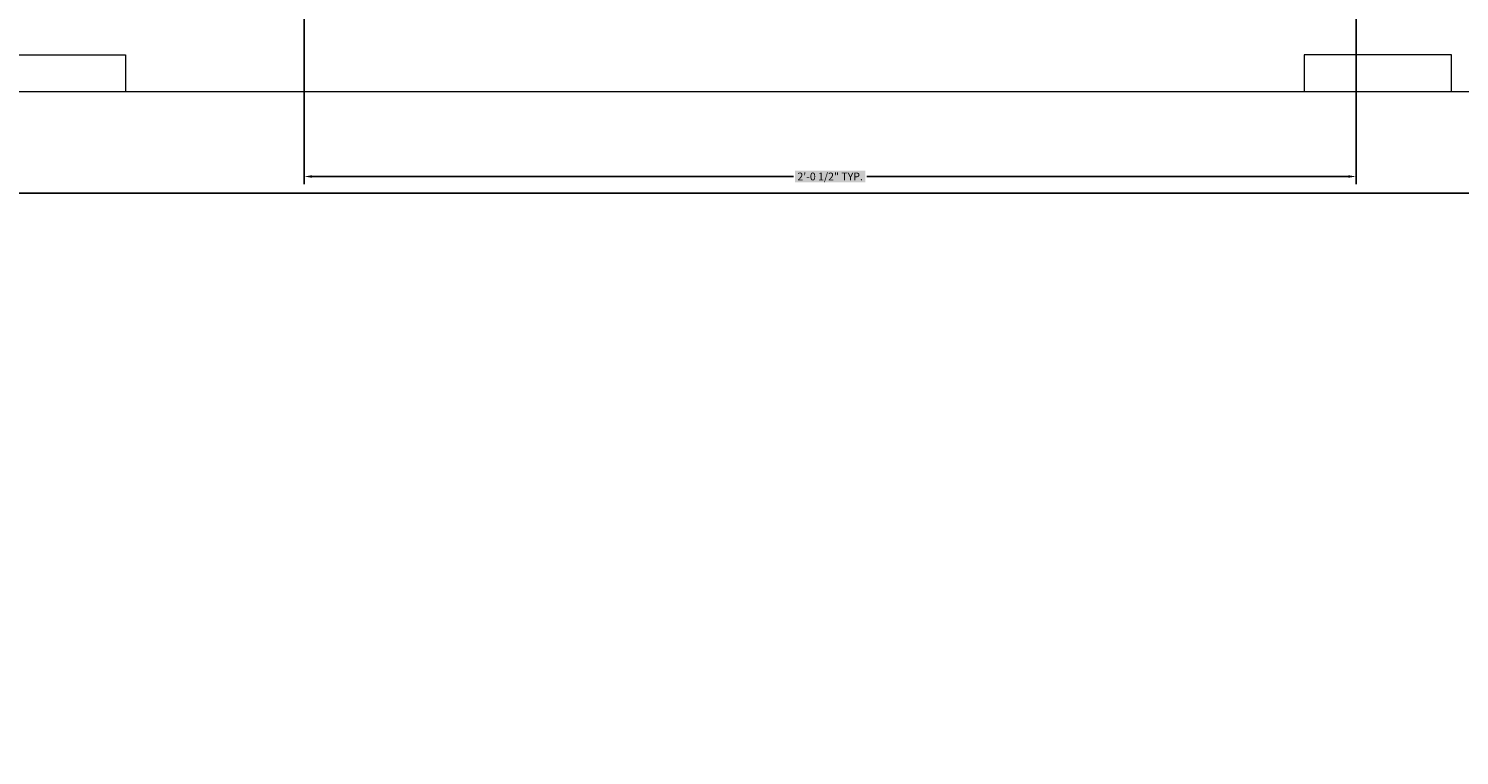
# Model space of a CAD drawing. Units: inches. Extents: x -301 to 715, y -607 to 364.
# Tile 79 of 141: x -94 to -61, y -56 to -39. Entities that reach past the tile are written whole.
import ezdxf

# ---------------------------------------------------------------- set-up
doc = ezdxf.new("R2010")
doc.units = ezdxf.units.IN
doc.header["$MEASUREMENT"] = 0
doc.layers.add('A-ANNO-DIMS', color=2, linetype='Continuous', lineweight=18)
doc.layers.add('A-FURN', color=8, linetype='Continuous', lineweight=18)
doc.styles.get("Standard").update_dxf_attribs({"font": 'arial.ttf'})
doc.dimstyles.get("Standard").update_dxf_attribs({"dimtxt": 0.18, "dimasz": 0.18, "dimexe": 0.18, "dimexo": 0.0625, "dimgap": 0.09, "dimtad": 0, "dimtih": 1, "dimtoh": 1, "dimdec": 1, "dimzin": 0, "dimdsep": 46, "dimlunit": 4, "dimtxsty": 'Standard', "dimcen": 0.09, "dimclrd": 3, "dimclre": 4, "dimclrt": 6, "dimadec": 0, "dimazin": 0, "dimtfac": 1, "dimtdec": 1, "dimtofl": 0, "dimtmove": 0, "dimatfit": 3, "dimfxl": 1, "dimtfill": 2, "dimtfillclr": 51, "dimtolj": 1, "dimtzin": 0, "dimarcsym": 0})

# ---------------------------------------------------------------- blocks, each defined once
blk = doc.blocks.new('Desk - 30 x 60 in.')
for p, q in [((26.999995, -30), (-26.999995, -30)), ((-16.000005, -31), (-16.000005, -30)), ((15.999995, -31), (15.999995, -30)), ((19.999995, -30), (19.999995, -31)), ((-20.000005, -31), (-16.000005, -31)), ((19.999995, -31), (15.999995, -31))]:
    blk.add_line(p, q)
blk = doc.blocks.new('*D57')
at = {"layer": 'A-ANNO-DIMS', "color": 0, "lineweight": -2, "transparency": 16777216}
for p, q in [((-195.603, -67.255), (-195.603, -42.99)), ((-190.603, -43.17), (-126.098, -43.17)), ((-56.603, -43.17), (-121.109, -43.17)), ((-51.603, -67.255), (-51.603, -42.99))]:
    blk.add_line(p, q, dxfattribs=at)
at = {"layer": 'A-ANNO-DIMS', "color": 0, "transparency": 16777216}
for points in [[(-190.603, -42.336), (-190.603, -44.003), (-195.603, -43.17)], [(-56.603, -42.336), (-56.603, -44.003), (-51.603, -43.17)]]:
    blk.add_solid(points, dxfattribs=at)
at = {"layer": 'Defpoints', "color": 0, "transparency": 16777216}
for p in [(-51.603, -43.17), (-195.603, -67.318), (-51.603, -67.318)]:
    blk.add_point(p, dxfattribs=at)
at = {"layer": 'A-ANNO-DIMS', "color": 0, "transparency": 16777216, "insert": (-123.603, -43.17), "char_height": 3, "attachment_point": 5, "bg_fill": 1, "box_fill_scale": 1.25, "bg_fill_color": 51, "bg_fill_transparency": 0}
blk.add_mtext("\\A1;12'", dxfattribs=at)
blk = doc.blocks.new('*D114')
at = {"layer": 'A-ANNO-DIMS', "color": 4, "lineweight": -2, "transparency": 16777216}
for p, q in [((-103.477, -39.895), (-103.477, -32.076)), ((-52.128, -39.895), (-52.128, -32.076))]:
    blk.add_line(p, q, dxfattribs=at)
at = {"layer": 'A-ANNO-DIMS', "color": 3, "lineweight": -2, "transparency": 16777216}
for p, q in [((-103.297, -32.256), (-79.024, -32.256)), ((-52.308, -32.256), (-76.581, -32.256))]:
    blk.add_line(p, q, dxfattribs=at)
at = {"layer": 'A-ANNO-DIMS', "color": 3, "transparency": 16777216}
for points in [[(-103.297, -32.226), (-103.297, -32.286), (-103.477, -32.256)], [(-52.308, -32.226), (-52.308, -32.286), (-52.128, -32.256)]]:
    blk.add_solid(points, dxfattribs=at)
at = {"layer": 'Defpoints', "color": 0, "transparency": 16777216}
for p in [(-52.128, -32.256), (-103.477, -39.958), (-52.128, -39.958)]:
    blk.add_point(p, dxfattribs=at)
at = {"layer": 'A-ANNO-DIMS', "color": 6, "transparency": 16777216, "insert": (-77.803, -32.256), "char_height": 0.18, "attachment_point": 5, "bg_fill": 1, "box_fill_scale": 1.25, "bg_fill_color": 51, "bg_fill_transparency": 0}
blk.add_mtext('\\A1;DESK 4\'-3 1/2" TYP.', dxfattribs=at)
blk = doc.blocks.new('*D117')
at = {"layer": 'A-ANNO-DIMS', "color": 4, "lineweight": -2, "transparency": 16777216}
for p, q in [((-87.341, -38.796), (-87.341, -42.963)), ((-62.906, -38.796), (-62.906, -42.963))]:
    blk.add_line(p, q, dxfattribs=at)
at = {"layer": 'A-ANNO-DIMS', "color": 3, "lineweight": -2, "transparency": 16777216}
for p, q in [((-87.161, -42.783), (-75.974, -42.783)), ((-63.086, -42.783), (-74.274, -42.783))]:
    blk.add_line(p, q, dxfattribs=at)
at = {"layer": 'A-ANNO-DIMS', "color": 3, "transparency": 16777216}
for points in [[(-87.161, -42.753), (-87.161, -42.813), (-87.341, -42.783)], [(-63.086, -42.753), (-63.086, -42.813), (-62.906, -42.783)]]:
    blk.add_solid(points, dxfattribs=at)
at = {"layer": 'Defpoints', "color": 0, "transparency": 16777216}
for p in [(-87.341, -38.733), (-62.906, -38.733), (-87.341, -42.783)]:
    blk.add_point(p, dxfattribs=at)
at = {"layer": 'A-ANNO-DIMS', "color": 6, "transparency": 16777216, "insert": (-75.124, -42.783), "char_height": 0.18, "attachment_point": 5, "bg_fill": 1, "box_fill_scale": 1.25, "bg_fill_color": 51, "bg_fill_transparency": 0}
blk.add_mtext('\\A1;2\'-0 1/2" TYP.', dxfattribs=at)
blk = doc.blocks.new('*D151')
at = {"layer": 'A-ANNO-DIMS', "color": 4, "lineweight": -2, "transparency": 16777216}
for p, q in [((-204.603, -223.755), (-204.603, 359.612)), ((-45.603, -214.755), (-45.603, 359.612))]:
    blk.add_line(p, q, dxfattribs=at)
at = {"layer": 'A-ANNO-DIMS', "color": 3, "lineweight": -2, "transparency": 16777216}
for p, q in [((-204.423, 359.432), (-125.494, 359.432)), ((-45.783, 359.432), (-124.713, 359.432))]:
    blk.add_line(p, q, dxfattribs=at)
at = {"layer": 'A-ANNO-DIMS', "color": 3, "transparency": 16777216}
for points in [[(-204.423, 359.462), (-204.423, 359.402), (-204.603, 359.432)], [(-45.783, 359.462), (-45.783, 359.402), (-45.603, 359.432)]]:
    blk.add_solid(points, dxfattribs=at)
at = {"layer": 'Defpoints', "color": 0, "transparency": 16777216}
for p in [(-45.603, 359.432), (-45.603, -214.818), (-204.603, -223.818)]:
    blk.add_point(p, dxfattribs=at)
at = {"layer": 'A-ANNO-DIMS', "color": 6, "transparency": 16777216, "insert": (-125.103, 359.432), "char_height": 0.18, "attachment_point": 5, "bg_fill": 1, "box_fill_scale": 1.25, "bg_fill_color": 51, "bg_fill_transparency": 0}
blk.add_mtext('\\A1;13\'-3"', dxfattribs=at)
blk = doc.blocks.new('*D158')
at = {"layer": 'A-ANNO-DIMS', "color": 4, "lineweight": -2, "transparency": 16777216}
for p, q in [((-122.603, 221.62), (-122.603, -296.865)), ((-50.603, 221.62), (-50.603, -296.865))]:
    blk.add_line(p, q, dxfattribs=at)
at = {"layer": 'A-ANNO-DIMS', "color": 3, "lineweight": -2, "transparency": 16777216}
for p, q in [((-122.423, -296.685), (-86.933, -296.685)), ((-50.783, -296.685), (-86.274, -296.685))]:
    blk.add_line(p, q, dxfattribs=at)
at = {"layer": 'A-ANNO-DIMS', "color": 3, "transparency": 16777216}
for points in [[(-122.423, -296.655), (-122.423, -296.715), (-122.603, -296.685)], [(-50.783, -296.655), (-50.783, -296.715), (-50.603, -296.685)]]:
    blk.add_solid(points, dxfattribs=at)
at = {"layer": 'Defpoints', "color": 0, "transparency": 16777216}
for p in [(-122.603, 221.682), (-50.603, 221.682), (-50.603, -296.685)]:
    blk.add_point(p, dxfattribs=at)
at = {"layer": 'A-ANNO-DIMS', "color": 6, "transparency": 16777216, "insert": (-86.603, -296.685), "char_height": 0.18, "attachment_point": 5, "bg_fill": 1, "box_fill_scale": 1.25, "bg_fill_color": 51, "bg_fill_transparency": 0}
blk.add_mtext('\\A1;6\'-0"', dxfattribs=at)

msp = doc.modelspace()

# ---------------------------------------------------------------- block references
at = {"layer": 'A-FURN', "xscale": -0.8558048107780498, "yscale": 0.8558048107780498, "zscale": 0.8558048107780498, "rotation": 180}
msp.add_blockref('Desk - 30 x 60 in.', (-77.803, -66.488), dxfattribs=at)

# ---------------------------------------------------------------- dimensions: what is measured, and where the dimension line sits
at = {"layer": 'A-ANNO-DIMS'}
for base, p1, p2, override, picture, middle in [((-45.603, 359.432), (-204.603, -223.818), (-45.603, -214.818), {"dimdec": 1, "dimlfac": 1, "dimrnd": 0, "dimzin": 1, "dimdsep": 46, "dimlunit": 4, "dimfrac": 2}, '*D151', (-125.103, 359.432)), ((-50.603, -296.685), (-122.603, 221.682), (-50.603, 221.682), {"dimdec": 1, "dimlfac": 1, "dimrnd": 0, "dimzin": 1, "dimdsep": 46, "dimlunit": 4, "dimfrac": 2}, '*D158', (-86.603, -296.685)), ((-51.603, -43.17), (-195.603, -67.318), (-51.603, -67.318), {"dimtxt": 3, "dimasz": 5, "dimclrd": 0, "dimclre": 0, "dimclrt": 0}, '*D57', (-123.603, -43.17))]:
    dim = msp.add_linear_dim(base=base, p1=p1, p2=p2, dimstyle='Standard', override=override, dxfattribs=at)
    dim.commit()
    dim.dimension.update_dxf_attribs({"geometry": picture, "text_midpoint": middle})
dim = msp.add_linear_dim(base=(-52.128, -32.256), p1=(-103.477, -39.958), p2=(-52.128, -39.958), text='DESK <> TYP.', dimstyle='Standard', override={"dimdec": 1, "dimlfac": 1, "dimrnd": 0, "dimzin": 1, "dimdsep": 46, "dimlunit": 4, "dimfrac": 2}, dxfattribs=at)
dim.commit()
dim.dimension.update_dxf_attribs({"geometry": '*D114', "text_midpoint": (-77.803, -32.256)})
dim = msp.add_linear_dim(base=(-87.341, -42.783), p1=(-62.906, -38.733), p2=(-87.341, -38.733), angle=180, text='<> TYP.', dimstyle='Standard', override={"dimdec": 1, "dimlfac": 1, "dimrnd": 0, "dimzin": 1, "dimdsep": 46, "dimlunit": 4, "dimfrac": 2}, dxfattribs=at)
dim.commit()
dim.dimension.update_dxf_attribs({"geometry": '*D117', "text_midpoint": (-75.124, -42.783)})

doc.saveas('drawing.dxf')
